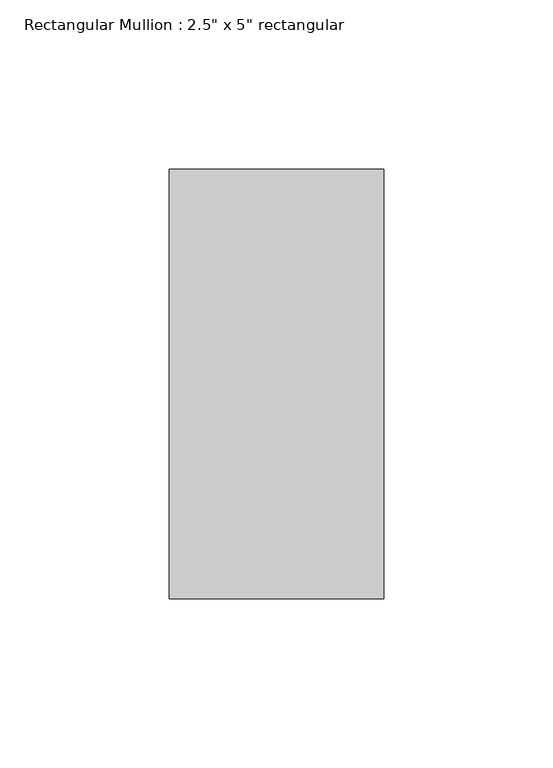
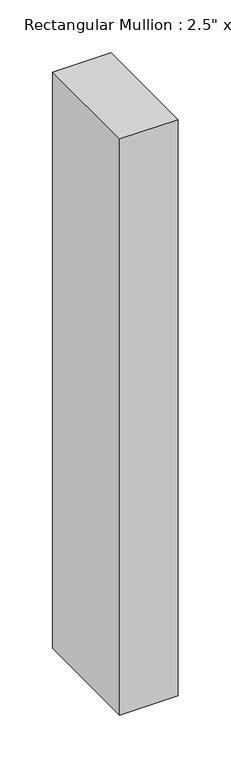
"""IFC4 building model written with IfcOpenShell, lengths in millimetres: member geometry."""

from ifc_helpers import new_model, si_unit, frame, origin, place, context, project, spatial, polyline, outline, extrude, source, transform, mapped, element, save


def member_e6bcc2de(model_context):
    return source(origin(), model_context, "Body", "SweptSolid", [
        extrude(outline(polyline([(0.0, 63.5), (0.0, -63.5), (-63.5, -63.5), (-63.5, 63.5), (0.0, 63.5)])), frame((0.0, 0.0, -665.4642589), z_axis=(0.0, 0.0, 1.0), x_axis=(1.0, 0.0, 0.0)), (0.0, 0.0, 1.0), 665.4642589),
    ])


if __name__ == "__main__":
    model = new_model("IFC4")
    model_context = context("Model", 3, world=origin())
    ifc_project = project(units=[si_unit("LENGTHUNIT", "METRE", prefix="MILLI")], contexts=[model_context])
    site = spatial("IfcSite", under=ifc_project)
    building = spatial("IfcBuilding", under=site)
    placement = place(None, origin())
    member_shape = member_e6bcc2de(model_context)
    element("IfcMember", 1, ObjectType="Rectangular Mullion : 2.5\" x 5\" rectangular", at=placement, inside=building, context=model_context, shape_type="MappedRepresentation", body=[
        mapped(member_shape, transform((0.0, 0.0, 0.0), x_axis=(1.0, 0.0, 0.0), y_axis=(0.0, 1.0, 0.0), z_axis=(0.0, 0.0, 1.0))),
    ])
    save(model, "model.ifc")

# Revit data of these elements
# Type "Rectangular Mullion : 2.5\" x 5\" rectangular"
#   built-in parameter 1007304 = 0.416667 (stored number, unit not read)
#   built-in parameter 1007301 = 0.104167 (stored number, unit not read)
#   built-in parameter 1007300 = 0.104167 (stored number, unit not read)
# Element 1 (IfcMember, "Rectangular Mullion : 2.5\" x 5\" rectangular")
#   Materials on its faces: "Aluminum"
# Materials
#   "Aluminum": class "Metal", colour RGB 247 247 247, transparency 0, Description = "Aluminum 6061", Cost = 0
